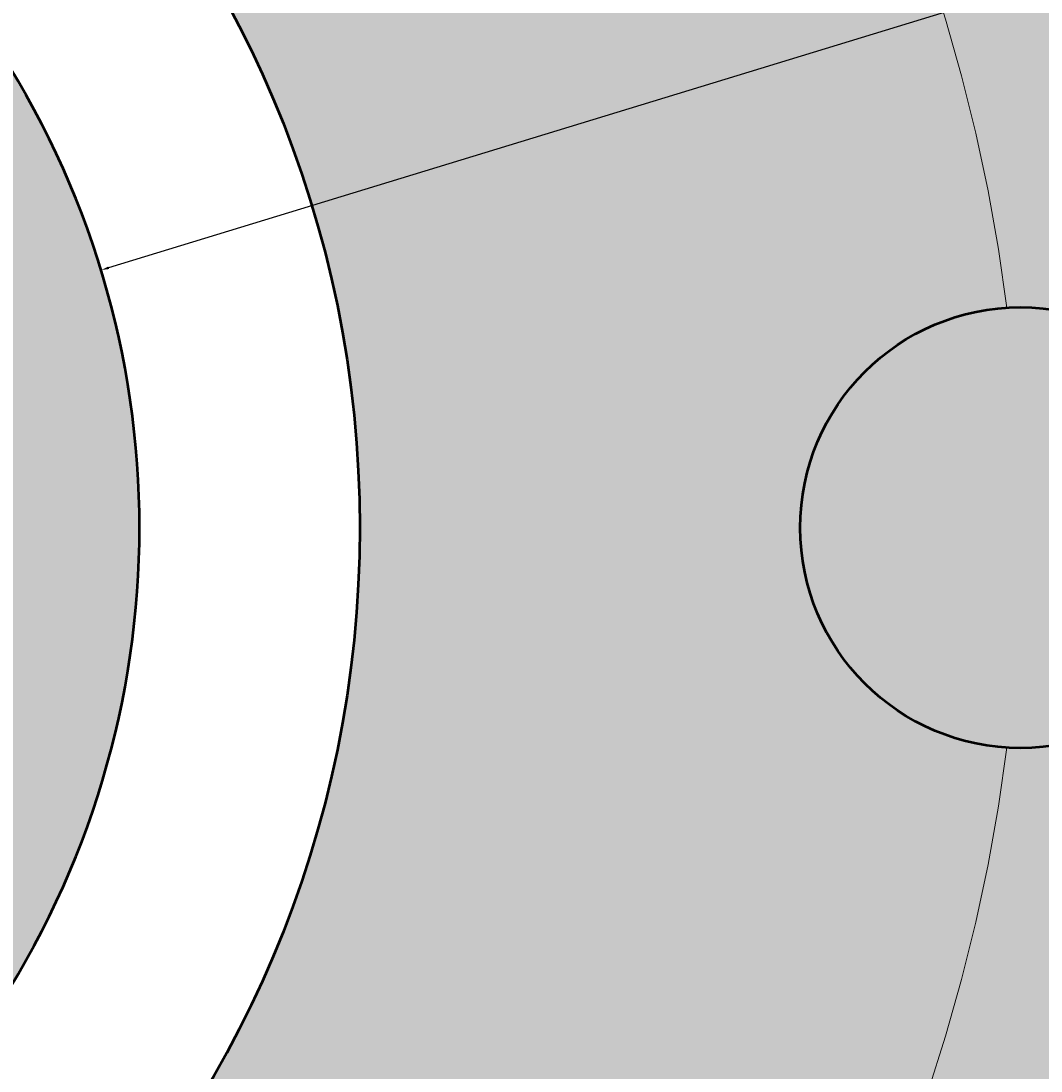
# Model space of a CAD drawing. Units: inches. Extents: x 139261 to 139415, y 52839 to 52963.
# Tile 15 of 20: x 139358 to 139381, y 52888 to 52912. Entities that reach past the tile are written whole.
import ezdxf

# ---------------------------------------------------------------- set-up
doc = ezdxf.new("R2010")
doc.units = ezdxf.units.IN
doc.header["$MEASUREMENT"] = 0
doc.linetypes.add('CENTER', pattern=[50.8, 31.75, -6.35, 6.35, -6.35])
for name, color, linetype, lineweight in [('M-CNTR', 4, 'CENTER', 18), ('M-DIMS', 2, 'Continuous', 25), ('M-HATC', 8, 'Continuous', 18), ('M-OUTL', 7, 'Continuous', 50)]:
    doc.layers.add(name, color=color, linetype=linetype, lineweight=lineweight)
doc.styles.get("Standard").update_dxf_attribs({"font": 'arial.ttf'})
doc.dimstyles.get("Standard").update_dxf_attribs({"dimtxt": 0.18, "dimasz": 0.18, "dimexe": 0.18, "dimexo": 0.0625, "dimgap": 0.09, "dimtad": 0, "dimtih": 1, "dimtoh": 1, "dimdec": 4, "dimzin": 0, "dimdsep": 46, "dimtxsty": 'Standard', "dimcen": 0.09, "dimadec": 0, "dimazin": 0, "dimtfac": 1, "dimtdec": 4, "dimtofl": 0, "dimtmove": 0, "dimatfit": 3, "dimfxl": 1, "dimtolj": 1, "dimtzin": 0, "dimarcsym": 0})

# ---------------------------------------------------------------- blocks, each defined once
blk = doc.blocks.new('*U1')
blk.add_circle((0, 0), 5)
blk = doc.blocks.new('*U2')
at = {"layer": 'M-OUTL', "color": 0, "linetype": 'ByBlock', "lineweight": -2, "transparency": 16777216, "rotation": 270}
blk.add_blockref('*U1', (139380.357, 52900.217), dxfattribs=at)
blk = doc.blocks.new('*D3')
at = {"layer": 'Defpoints', "color": 0, "transparency": 16777216}
for p in [(139359.484, 52906.062), (139321.23, 52894.373)]:
    blk.add_point(p, dxfattribs=at)
at = {"layer": 'M-DIMS', "color": 0, "lineweight": -2, "transparency": 16777216}
for p, q in [((139412.091, 52922.136), (139359.656, 52906.115)), ((139412.271, 52922.136), (139412.091, 52922.136)), ((139340.267, 52900.217), (139340.447, 52900.217)), ((139340.357, 52900.127), (139340.357, 52900.307))]:
    blk.add_line(p, q, dxfattribs=at)
at = {"layer": 'M-DIMS', "color": 0, "transparency": 16777216}
blk.add_solid([(139359.647, 52906.143), (139359.665, 52906.086), (139359.484, 52906.062)], dxfattribs=at)
at = {"layer": 'M-DIMS', "color": 0, "transparency": 16777216, "insert": (139412.902, 52922.136), "char_height": 0.18, "attachment_point": 5}
blk.add_mtext('\\A1;∅40.0000', dxfattribs=at)
blk = doc.blocks.new('*D4')
at = {"layer": 'Defpoints', "color": 0, "transparency": 16777216}
for p in [(139373.053, 52923.26), (139307.661, 52877.175)]:
    blk.add_point(p, dxfattribs=at)
at = {"layer": 'M-DIMS', "color": 0, "lineweight": -2, "transparency": 16777216}
for p, q in [((139414.011, 52952.126), (139373.2, 52923.364)), ((139414.191, 52952.126), (139414.011, 52952.126)), ((139340.267, 52900.217), (139340.447, 52900.217)), ((139340.357, 52900.127), (139340.357, 52900.307))]:
    blk.add_line(p, q, dxfattribs=at)
blk.add_arc((139340.357, 52900.217), 40, 34.9168, 52.0771, dxfattribs=at)
at = {"layer": 'M-DIMS', "color": 0, "transparency": 16777216}
blk.add_solid([(139373.183, 52923.388), (139373.217, 52923.339), (139373.053, 52923.26)], dxfattribs=at)
at = {"layer": 'M-DIMS', "color": 0, "transparency": 16777216, "insert": (139414.822, 52952.126), "char_height": 0.18, "attachment_point": 5}
blk.add_mtext('\\A1;∅80.0000', dxfattribs=at)
blk = doc.blocks.new('*D5')
at = {"layer": 'Defpoints', "color": 0, "transparency": 16777216}
for p in [(139316.763, 52908.484), (139363.951, 52891.951)]:
    blk.add_point(p, dxfattribs=at)
at = {"layer": 'M-DIMS', "color": 0, "lineweight": -2, "transparency": 16777216}
for p, q in [((139262.553, 52927.414), (139262.733, 52927.414)), ((139262.733, 52927.414), (139316.593, 52908.544)), ((139340.267, 52900.217), (139340.447, 52900.217)), ((139340.357, 52900.127), (139340.357, 52900.307))]:
    blk.add_line(p, q, dxfattribs=at)
at = {"layer": 'M-DIMS', "color": 0, "transparency": 16777216}
blk.add_solid([(139316.603, 52908.572), (139316.583, 52908.515), (139316.763, 52908.484)], dxfattribs=at)
at = {"layer": 'M-DIMS', "color": 0, "transparency": 16777216, "insert": (139261.922, 52927.414), "char_height": 0.18, "attachment_point": 5}
blk.add_mtext('\\A1;∅50.0000', dxfattribs=at)
blk = doc.blocks.new('*D9')
at = {"layer": 'Defpoints', "color": 0, "transparency": 16777216}
for p in [(139302.054, 52932.357), (139378.659, 52868.078)]:
    blk.add_point(p, dxfattribs=at)
at = {"layer": 'M-DIMS', "color": 0, "lineweight": -2, "transparency": 16777216}
for p, q in [((139278.893, 52951.64), (139279.073, 52951.64)), ((139279.073, 52951.64), (139301.916, 52932.472)), ((139340.267, 52900.217), (139340.447, 52900.217)), ((139340.357, 52900.127), (139340.357, 52900.307))]:
    blk.add_line(p, q, dxfattribs=at)
at = {"layer": 'M-DIMS', "color": 0, "transparency": 16777216}
blk.add_solid([(139301.936, 52932.495), (139301.897, 52932.449), (139302.054, 52932.357)], dxfattribs=at)
at = {"layer": 'M-DIMS', "color": 0, "transparency": 16777216, "insert": (139278.506, 52951.64), "char_height": 0.18, "attachment_point": 5}
blk.add_mtext('\\A1;∅100', dxfattribs=at)
blk = doc.blocks.new('*D10')
at = {"layer": 'Defpoints', "color": 0, "transparency": 16777216}
for p in [(139325.07, 52937.181), (139355.644, 52863.254)]:
    blk.add_point(p, dxfattribs=at)
at = {"layer": 'M-DIMS', "color": 0, "lineweight": -2, "transparency": 16777216}
for p, q in [((139340.267, 52900.217), (139340.447, 52900.217)), ((139340.357, 52900.127), (139340.357, 52900.307)), ((139364.816, 52841.075), (139355.712, 52863.087)), ((139364.996, 52841.075), (139364.816, 52841.075))]:
    blk.add_line(p, q, dxfattribs=at)
at = {"layer": 'M-DIMS', "color": 0, "transparency": 16777216}
blk.add_solid([(139355.74, 52863.099), (139355.685, 52863.076), (139355.644, 52863.254)], dxfattribs=at)
at = {"layer": 'M-DIMS', "color": 0, "transparency": 16777216, "insert": (139365.312, 52841.075), "char_height": 0.18, "attachment_point": 5}
blk.add_mtext('\\A1;∅80', dxfattribs=at)

msp = doc.modelspace()

# ---------------------------------------------------------------- hatches: boundary and pattern name
at = {"layer": 'M-HATC'}
h = msp.add_hatch(color=256, dxfattribs=at)
h.dxf.hatch_style = 1
h.paths.add_polyline_path([(139290.35689, 52900.21749, 1), (139390.35689, 52900.21749, 1)])
h.paths.add_polyline_path([(139335.36666, 52939.90499, -0.01563646), (139335.35689, 52940.21749, -1), (139345.35689, 52940.21749, -0.01563646), (139345.34711, 52939.90499, -0.13461315), (139364.89157, 52931.80941, -0.691035), (139373.64116, 52928.50176, -0.21521822), (139371.94881, 52924.75216, -0.13461315), (139380.04439, 52905.20771, -0.43265224), (139385.35689, 52900.21749, -0.43265224), (139380.04439, 52895.22726, -0.13461315), (139371.94881, 52875.68281, -0.21521822), (139373.64116, 52871.93321, -0.691035), (139364.89157, 52868.62556, -0.13461315), (139345.34711, 52860.52999, -0.01563646), (139345.35689, 52860.21749, -1), (139335.35689, 52860.21749, -0.01563646), (139335.36666, 52860.52999, -0.13461315), (139315.82221, 52868.62556, -0.691035), (139307.07262, 52871.93321, -0.21521822), (139308.76496, 52875.68281, -0.13461315), (139300.66939, 52895.22726, -0.43265224), (139295.35689, 52900.21749, -0.43265224), (139300.66939, 52905.20771, -0.13461315), (139308.76496, 52924.75216, -0.21521822), (139307.07262, 52928.50176, -0.691035), (139315.82221, 52931.80941, -0.13461315)], flags=16)
h.paths.add_polyline_path([(139365.35689, 52900.21749, -1), (139315.35689, 52900.21749, -1)], flags=0)
h.paths.add_polyline_path([(139323.71474, 52911.30978), (139356.99903, 52911.30978, -0.3027197), (139356.99903, 52889.12519), (139323.71474, 52889.12519, -0.3027197)], flags=0)
h.paths.add_polyline_path([(139364.89157, 52931.80941, 0.13461315), (139345.34711, 52939.90499, -0.93933644), (139335.36666, 52939.90499, 0.13461315), (139315.82221, 52931.80941, -0.18270763), (139317.07262, 52928.50176, -0.64579494), (139308.76496, 52924.75216, 0.13461315), (139300.66939, 52905.20771, -0.39601219), (139305.35689, 52900.21749, -0.39601219), (139300.66939, 52895.22726, 0.13461315), (139308.76496, 52875.68281, -0.64579494), (139317.07262, 52871.93321, -0.18270763), (139315.82221, 52868.62556, 0.13461315), (139335.36666, 52860.52999, -0.93933644), (139345.34711, 52860.52999, 0.13461315), (139364.89157, 52868.62556, -0.18270763), (139363.64116, 52871.93321, -0.64579494), (139371.94881, 52875.68281, 0.13461315), (139380.04439, 52895.22726, -0.39601219), (139375.35689, 52900.21749, -0.39601219), (139380.04439, 52905.20771, 0.13461315), (139371.94881, 52924.75216, -0.64579494), (139363.64116, 52928.50176, -0.18270763)], flags=0)
h = msp.add_hatch(color=256, dxfattribs=at)
h.dxf.hatch_style = 1
h.set_gradient(color1=(205, 105, 40), tint=1)
h.paths.add_polyline_path([(139335.35689, 52940.21749, 1), (139345.35689, 52940.21749, 1)])
h.paths.add_polyline_path([(139307.07262, 52928.50176, 1), (139317.07262, 52928.50176, 1)])
h.paths.add_polyline_path([(139295.35689, 52900.21749, 1), (139305.35689, 52900.21749, 1)])
h.paths.add_polyline_path([(139307.07262, 52871.93321, 1), (139317.07262, 52871.93321, 1)])
h.paths.add_polyline_path([(139345.35689, 52860.21749, 1), (139335.35689, 52860.21749, 1)])
h.paths.add_polyline_path([(139363.64116, 52871.93321, 1), (139373.64116, 52871.93321, 1)])
h.paths.add_polyline_path([(139375.35689, 52900.21749, 1), (139385.35689, 52900.21749, 1)])
h.paths.add_polyline_path([(139363.64116, 52928.50176, 1), (139373.64116, 52928.50176, 1)])
h = msp.add_hatch(color=256, dxfattribs=at)
h.dxf.hatch_style = 1
h.paths.add_polyline_path([(139345.34711, 52939.90499, -0.93933644), (139335.36666, 52939.90499, 0.13461315), (139315.82221, 52931.80941, -0.18270763), (139317.07262, 52928.50176, -0.64579494), (139308.76496, 52924.75216, 0.13461315), (139300.66939, 52905.20771, -0.39601219), (139305.35689, 52900.21749, -0.39601219), (139300.66939, 52895.22726, 0.13461315), (139308.76496, 52875.68281, -0.64579494), (139317.07262, 52871.93321, -0.18270763), (139315.82221, 52868.62556, 0.13461315), (139335.36666, 52860.52999, -0.93933644), (139345.34711, 52860.52999, 0.13461315), (139364.89157, 52868.62556, -0.18270763), (139363.64116, 52871.93321, -0.64579494), (139371.94881, 52875.68281, 0.13461315), (139380.04439, 52895.22726, -0.39601219), (139375.35689, 52900.21749, -0.39601219), (139380.04439, 52905.20771, 0.13461315), (139371.94881, 52924.75216, -0.64579494), (139363.64116, 52928.50176, -0.18270763), (139364.89157, 52931.80941, 0.13461315)])
h.paths.add_polyline_path([(139365.35689, 52900.21749, -1), (139315.35689, 52900.21749, -1)], flags=16)
h.paths.add_polyline_path([(139356.99903, 52911.30978, -0.3027197), (139356.99903, 52889.12519), (139323.71474, 52889.12519, -0.3027197), (139323.71474, 52911.30978)], flags=0)
h = msp.add_hatch(color=256, dxfattribs=at)
h.dxf.hatch_style = 1
h.paths.add_polyline_path([(139356.99903, 52911.30978), (139323.71474, 52911.30978, 0.3027197), (139323.71474, 52889.12519), (139356.99903, 52889.12519, 0.3027197)])

# ---------------------------------------------------------------- linework, layer by layer
at = {"layer": 'M-CNTR'}
for start, end in [(7.166643, 37.833357), (322.166643, 352.833357)]:
    msp.add_arc((139340.35689, 52900.21749), 40, start, end, dxfattribs=at)
at = {"layer": 'M-OUTL'}
for radius in [50, 25]:
    msp.add_circle((139340.35689, 52900.21749), radius, dxfattribs=at)
msp.add_arc((139340.35689, 52900.21749), 20, 326.315805, 33.684195, dxfattribs=at)

# ---------------------------------------------------------------- block references
msp.add_blockref('*U2', (0, 0), dxfattribs=at)

# ---------------------------------------------------------------- dimensions: what is measured, and where the dimension line sits
at = {"layer": 'M-DIMS'}
for p1, p2, override, picture, middle in [((139307.66087, 52877.17469), (139373.0529, 52923.26028), {"dimclrd": 0, "dimclre": 0, "dimclrt": 0}, '*D4', (139414.82217, 52952.12585)), ((139378.65939, 52868.07845), (139302.05438, 52932.35652), {"dimdec": 0, "dimlfac": 1, "dimrnd": 0, "dimzin": 0, "dimdsep": 46, "dimlunit": 2}, '*D9', (139278.50641, 52951.63995)), ((139325.07023, 52937.18123), (139355.64354, 52863.25374), {"dimdec": 0, "dimlfac": 1, "dimrnd": 0, "dimzin": 0, "dimdsep": 46, "dimlunit": 2}, '*D10', (139365.31206, 52841.0755)), ((139363.95063, 52891.95098), (139316.76314, 52908.48399), {"dimclrd": 0, "dimclre": 0, "dimclrt": 0}, '*D5', (139261.92224, 52927.41429)), ((139321.22987, 52894.37307), (139359.4839, 52906.0619), {"dimclrd": 0, "dimclre": 0, "dimclrt": 0}, '*D3', (139412.90184, 52922.13633))]:
    dim = msp.add_diameter_dim_2p(p1=p1, p2=p2, dimstyle='Standard', override=override, dxfattribs=at)
    dim.commit()
    dim.dimension.update_dxf_attribs({"geometry": picture, "text_midpoint": middle, "dimtype": 163})

doc.saveas('drawing.dxf')
